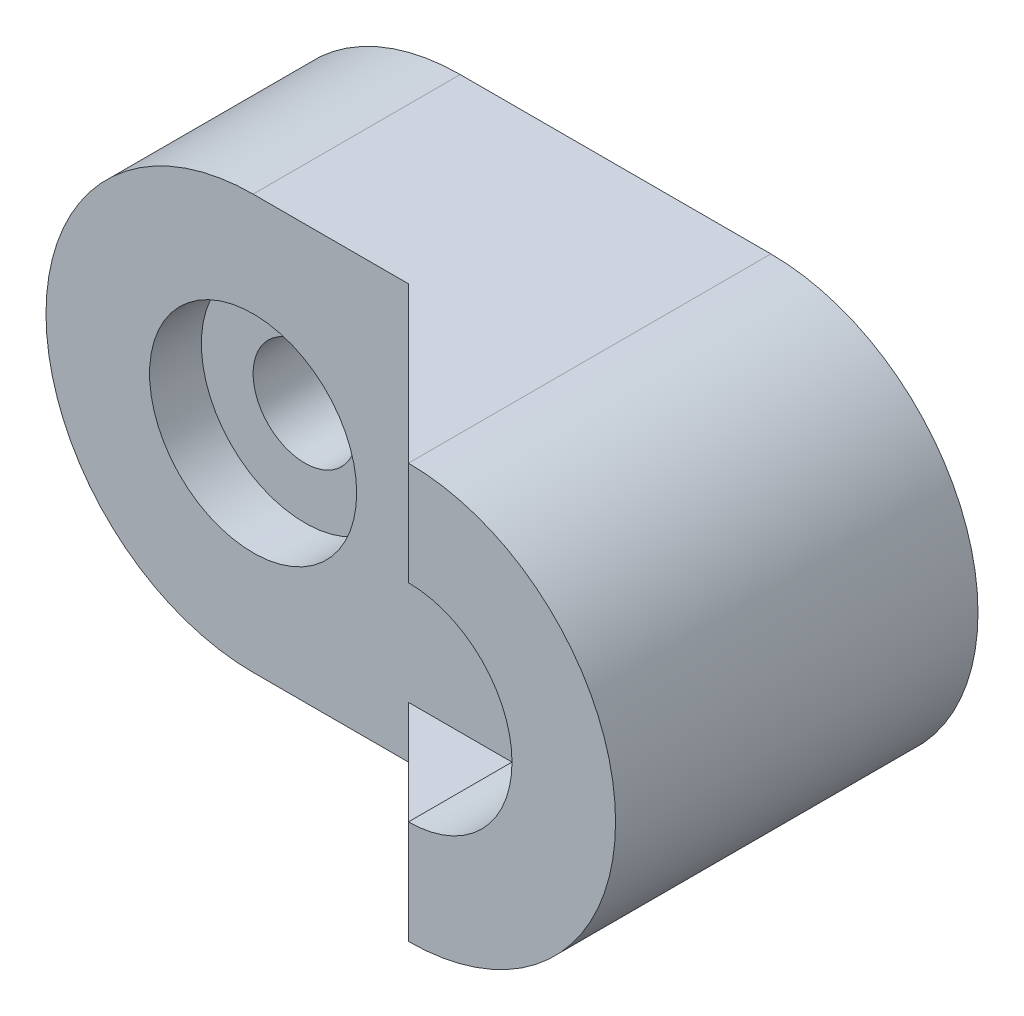
ISO-10303-21;
HEADER;
FILE_DESCRIPTION(('STEP AP214'),'2;1');
FILE_NAME('part.step','',(''),(''),'','','');
FILE_SCHEMA(('AUTOMOTIVE_DESIGN { 1 0 10303 214 1 1 1 1 }'));
ENDSEC;
DATA;
#1=APPLICATION_CONTEXT('core data for automotive mechanical design processes');
#2=APPLICATION_PROTOCOL_DEFINITION('international standard','automotive_design',2000,#1);
#3=PRODUCT_CONTEXT('',#1,'mechanical');
#4=PRODUCT('Part','Part','',(#3));
#5=PRODUCT_RELATED_PRODUCT_CATEGORY('part','',(#4));
#6=PRODUCT_DEFINITION_FORMATION('','',#4);
#7=PRODUCT_DEFINITION_CONTEXT('part definition',#1,'design');
#8=PRODUCT_DEFINITION('design','',#6,#7);
#9=PRODUCT_DEFINITION_SHAPE('','',#8);
#10=(LENGTH_UNIT() NAMED_UNIT(*) SI_UNIT(.MILLI.,.METRE.));
#11=(NAMED_UNIT(*) PLANE_ANGLE_UNIT() SI_UNIT($,.RADIAN.));
#12=(NAMED_UNIT(*) SI_UNIT($,.STERADIAN.) SOLID_ANGLE_UNIT());
#13=UNCERTAINTY_MEASURE_WITH_UNIT(LENGTH_MEASURE(1.E-05),#10,'distance_accuracy_value','');
#14=(GEOMETRIC_REPRESENTATION_CONTEXT(3) GLOBAL_UNCERTAINTY_ASSIGNED_CONTEXT((#13)) GLOBAL_UNIT_ASSIGNED_CONTEXT((#10,
#11,#12)) REPRESENTATION_CONTEXT('',''));
#15=CARTESIAN_POINT('',(0.,0.,0.));
#16=DIRECTION('',(0.,0.,1.));
#17=DIRECTION('',(1.,0.,0.));
#18=AXIS2_PLACEMENT_3D('',#15,#16,#17);
#19=CARTESIAN_POINT('',(60.,40.,70.));
#20=DIRECTION('',(1.,0.,0.));
#21=DIRECTION('',(0.,1.,0.));
#22=AXIS2_PLACEMENT_3D('',#19,#20,#21);
#23=PLANE('',#22);
#24=DIRECTION('',(0.,0.,-1.));
#25=VECTOR('',#24,1.);
#26=CARTESIAN_POINT('',(60.,30.,70.));
#27=LINE('',#26,#25);
#28=CARTESIAN_POINT('',(60.,30.,70.));
#29=VERTEX_POINT('',#28);
#30=CARTESIAN_POINT('',(60.,30.,40.));
#31=VERTEX_POINT('',#30);
#32=EDGE_CURVE('E127',#29,#31,#27,.T.);
#33=ORIENTED_EDGE('',*,*,#32,.T.);
#34=DIRECTION('',(0.,-1.,0.));
#35=VECTOR('',#34,1.);
#36=CARTESIAN_POINT('',(60.,40.,40.));
#37=LINE('',#36,#35);
#38=CARTESIAN_POINT('',(60.,20.,40.));
#39=VERTEX_POINT('',#38);
#40=EDGE_CURVE('E132',#31,#39,#37,.T.);
#41=ORIENTED_EDGE('',*,*,#40,.T.);
#42=DIRECTION('',(0.,0.,1.));
#43=VECTOR('',#42,1.);
#44=CARTESIAN_POINT('',(60.,20.,40.));
#45=LINE('',#44,#43);
#46=CARTESIAN_POINT('',(60.,20.,70.));
#47=VERTEX_POINT('',#46);
#48=EDGE_CURVE('E241',#39,#47,#45,.T.);
#49=ORIENTED_EDGE('',*,*,#48,.T.);
#50=DIRECTION('',(0.,-1.,0.));
#51=VECTOR('',#50,1.);
#52=CARTESIAN_POINT('',(60.,40.,70.));
#53=LINE('',#52,#51);
#54=EDGE_CURVE('E140',#29,#47,#53,.T.);
#55=ORIENTED_EDGE('',*,*,#54,.F.);
#56=EDGE_LOOP('',(#33,#41,#49,#55));
#57=FACE_BOUND('',#56,.T.);
#58=ADVANCED_FACE('F44',(#57),#23,.F.);
#59=CARTESIAN_POINT('',(0.,0.,40.));
#60=DIRECTION('',(0.,0.,-1.));
#61=DIRECTION('',(-1.,0.,0.));
#62=AXIS2_PLACEMENT_3D('',#59,#60,#61);
#63=CYLINDRICAL_SURFACE('',#62,40.);
#64=CARTESIAN_POINT('',(0.,0.,0.));
#65=DIRECTION('',(0.,0.,1.));
#66=DIRECTION('',(1.,0.,0.));
#67=AXIS2_PLACEMENT_3D('',#64,#65,#66);
#68=CIRCLE('',#67,40.);
#69=CARTESIAN_POINT('',(0.,40.,0.));
#70=VERTEX_POINT('',#69);
#71=CARTESIAN_POINT('',(0.,-40.,0.));
#72=VERTEX_POINT('',#71);
#73=EDGE_CURVE('E164',#70,#72,#68,.T.);
#74=ORIENTED_EDGE('',*,*,#73,.T.);
#75=DIRECTION('',(0.,0.,-1.));
#76=VECTOR('',#75,1.);
#77=CARTESIAN_POINT('',(0.,-40.,40.));
#78=LINE('',#77,#76);
#79=CARTESIAN_POINT('',(0.,-40.,40.));
#80=VERTEX_POINT('',#79);
#81=EDGE_CURVE('E11',#80,#72,#78,.T.);
#82=ORIENTED_EDGE('',*,*,#81,.F.);
#83=CARTESIAN_POINT('',(0.,0.,40.));
#84=DIRECTION('',(0.,0.,1.));
#85=DIRECTION('',(1.,0.,0.));
#86=AXIS2_PLACEMENT_3D('',#83,#84,#85);
#87=CIRCLE('',#86,40.);
#88=CARTESIAN_POINT('',(0.,40.,40.));
#89=VERTEX_POINT('',#88);
#90=EDGE_CURVE('E166',#89,#80,#87,.T.);
#91=ORIENTED_EDGE('',*,*,#90,.F.);
#92=DIRECTION('',(0.,0.,-1.));
#93=VECTOR('',#92,1.);
#94=CARTESIAN_POINT('',(0.,40.,40.));
#95=LINE('',#94,#93);
#96=EDGE_CURVE('E180',#89,#70,#95,.T.);
#97=ORIENTED_EDGE('',*,*,#96,.T.);
#98=EDGE_LOOP('',(#74,#82,#91,#97));
#99=FACE_BOUND('',#98,.T.);
#100=ADVANCED_FACE('F50',(#99),#63,.T.);
#101=CARTESIAN_POINT('',(60.,-40.,40.));
#102=DIRECTION('',(0.,1.,0.));
#103=DIRECTION('',(-1.,0.,0.));
#104=AXIS2_PLACEMENT_3D('',#101,#102,#103);
#105=PLANE('',#104);
#106=DIRECTION('',(1.,0.,0.));
#107=VECTOR('',#106,1.);
#108=CARTESIAN_POINT('',(60.,-40.,0.));
#109=LINE('',#108,#107);
#110=CARTESIAN_POINT('',(60.,-40.,0.));
#111=VERTEX_POINT('',#110);
#112=EDGE_CURVE('E179',#72,#111,#109,.T.);
#113=ORIENTED_EDGE('',*,*,#112,.T.);
#114=DIRECTION('',(0.,0.,-1.));
#115=VECTOR('',#114,1.);
#116=CARTESIAN_POINT('',(60.,-40.,40.));
#117=LINE('',#116,#115);
#118=CARTESIAN_POINT('',(60.,-40.,70.));
#119=VERTEX_POINT('',#118);
#120=EDGE_CURVE('E52',#119,#111,#117,.T.);
#121=ORIENTED_EDGE('',*,*,#120,.F.);
#122=DIRECTION('',(-0.707106781186547,0.,-0.707106781186548));
#123=VECTOR('',#122,1.);
#124=CARTESIAN_POINT('',(30.,-40.,40.));
#125=LINE('',#124,#123);
#126=CARTESIAN_POINT('',(30.,-40.,40.));
#127=VERTEX_POINT('',#126);
#128=EDGE_CURVE('E229',#119,#127,#125,.T.);
#129=ORIENTED_EDGE('',*,*,#128,.T.);
#130=DIRECTION('',(1.,0.,0.));
#131=VECTOR('',#130,1.);
#132=CARTESIAN_POINT('',(60.,-40.,40.));
#133=LINE('',#132,#131);
#134=EDGE_CURVE('E171',#80,#127,#133,.T.);
#135=ORIENTED_EDGE('',*,*,#134,.F.);
#136=ORIENTED_EDGE('',*,*,#81,.T.);
#137=EDGE_LOOP('',(#113,#121,#129,#135,#136));
#138=FACE_BOUND('',#137,.T.);
#139=ADVANCED_FACE('F257',(#138),#105,.F.);
#140=CARTESIAN_POINT('',(60.,0.,40.));
#141=DIRECTION('',(0.,0.,-1.));
#142=DIRECTION('',(-1.,0.,0.));
#143=AXIS2_PLACEMENT_3D('',#140,#141,#142);
#144=CYLINDRICAL_SURFACE('',#143,40.);
#145=CARTESIAN_POINT('',(60.,0.,0.));
#146=DIRECTION('',(0.,0.,1.));
#147=DIRECTION('',(1.,0.,0.));
#148=AXIS2_PLACEMENT_3D('',#145,#146,#147);
#149=CIRCLE('',#148,40.);
#150=CARTESIAN_POINT('',(60.,40.,0.));
#151=VERTEX_POINT('',#150);
#152=EDGE_CURVE('E185',#111,#151,#149,.T.);
#153=ORIENTED_EDGE('',*,*,#152,.T.);
#154=DIRECTION('',(0.,0.,-1.));
#155=VECTOR('',#154,1.);
#156=CARTESIAN_POINT('',(60.,40.,40.));
#157=LINE('',#156,#155);
#158=CARTESIAN_POINT('',(60.,40.,70.));
#159=VERTEX_POINT('',#158);
#160=EDGE_CURVE('E190',#159,#151,#157,.T.);
#161=ORIENTED_EDGE('',*,*,#160,.F.);
#162=CARTESIAN_POINT('',(60.,0.,70.));
#163=DIRECTION('',(0.,0.,1.));
#164=DIRECTION('',(1.,0.,0.));
#165=AXIS2_PLACEMENT_3D('',#162,#163,#164);
#166=CIRCLE('',#165,40.);
#167=EDGE_CURVE('E143',#119,#159,#166,.T.);
#168=ORIENTED_EDGE('',*,*,#167,.F.);
#169=ORIENTED_EDGE('',*,*,#120,.T.);
#170=EDGE_LOOP('',(#153,#161,#168,#169));
#171=FACE_BOUND('',#170,.T.);
#172=ADVANCED_FACE('F194',(#171),#144,.T.);
#173=CARTESIAN_POINT('',(0.,40.,40.));
#174=DIRECTION('',(0.,-1.,0.));
#175=DIRECTION('',(1.,0.,0.));
#176=AXIS2_PLACEMENT_3D('',#173,#174,#175);
#177=PLANE('',#176);
#178=DIRECTION('',(-1.,0.,0.));
#179=VECTOR('',#178,1.);
#180=CARTESIAN_POINT('',(0.,40.,0.));
#181=LINE('',#180,#179);
#182=EDGE_CURVE('E175',#151,#70,#181,.T.);
#183=ORIENTED_EDGE('',*,*,#182,.T.);
#184=ORIENTED_EDGE('',*,*,#96,.F.);
#185=DIRECTION('',(-1.,0.,0.));
#186=VECTOR('',#185,1.);
#187=CARTESIAN_POINT('',(0.,40.,40.));
#188=LINE('',#187,#186);
#189=CARTESIAN_POINT('',(30.,40.,40.));
#190=VERTEX_POINT('',#189);
#191=EDGE_CURVE('E174',#190,#89,#188,.T.);
#192=ORIENTED_EDGE('',*,*,#191,.F.);
#193=DIRECTION('',(0.707106781186547,0.,0.707106781186548));
#194=VECTOR('',#193,1.);
#195=CARTESIAN_POINT('',(30.,40.,40.));
#196=LINE('',#195,#194);
#197=EDGE_CURVE('E208',#190,#159,#196,.T.);
#198=ORIENTED_EDGE('',*,*,#197,.T.);
#199=ORIENTED_EDGE('',*,*,#160,.T.);
#200=EDGE_LOOP('',(#183,#184,#192,#198,#199));
#201=FACE_BOUND('',#200,.T.);
#202=ADVANCED_FACE('F203',(#201),#177,.F.);
#203=CARTESIAN_POINT('',(0.,0.,40.));
#204=DIRECTION('',(0.,0.,1.));
#205=DIRECTION('',(1.,0.,0.));
#206=AXIS2_PLACEMENT_3D('',#203,#204,#205);
#207=PLANE('',#206);
#208=DIRECTION('',(0.,1.,0.));
#209=VECTOR('',#208,1.);
#210=CARTESIAN_POINT('',(30.,30.,40.));
#211=LINE('',#210,#209);
#212=CARTESIAN_POINT('',(30.,30.,40.));
#213=VERTEX_POINT('',#212);
#214=EDGE_CURVE('E133',#213,#190,#211,.T.);
#215=ORIENTED_EDGE('',*,*,#214,.T.);
#216=ORIENTED_EDGE('',*,*,#191,.T.);
#217=ORIENTED_EDGE('',*,*,#90,.T.);
#218=ORIENTED_EDGE('',*,*,#134,.T.);
#219=DIRECTION('',(0.,-1.,0.));
#220=VECTOR('',#219,1.);
#221=CARTESIAN_POINT('',(30.,-30.,40.));
#222=LINE('',#221,#220);
#223=CARTESIAN_POINT('',(30.,-30.,40.));
#224=VERTEX_POINT('',#223);
#225=EDGE_CURVE('E225',#224,#127,#222,.T.);
#226=ORIENTED_EDGE('',*,*,#225,.F.);
#227=DIRECTION('',(1.,0.,0.));
#228=VECTOR('',#227,1.);
#229=CARTESIAN_POINT('',(60.,-30.,40.));
#230=LINE('',#229,#228);
#231=CARTESIAN_POINT('',(60.,-30.,40.));
#232=VERTEX_POINT('',#231);
#233=EDGE_CURVE('E249',#224,#232,#230,.T.);
#234=ORIENTED_EDGE('',*,*,#233,.T.);
#235=CARTESIAN_POINT('',(60.,-20.,40.));
#236=VERTEX_POINT('',#235);
#237=EDGE_CURVE('E147',#236,#232,#37,.T.);
#238=ORIENTED_EDGE('',*,*,#237,.F.);
#239=CARTESIAN_POINT('',(60.,0.,40.));
#240=DIRECTION('',(0.,0.,1.));
#241=DIRECTION('',(1.,0.,0.));
#242=AXIS2_PLACEMENT_3D('',#239,#240,#241);
#243=CIRCLE('',#242,20.);
#244=EDGE_CURVE('E141',#39,#236,#243,.T.);
#245=ORIENTED_EDGE('',*,*,#244,.F.);
#246=ORIENTED_EDGE('',*,*,#40,.F.);
#247=DIRECTION('',(-1.,0.,0.));
#248=VECTOR('',#247,1.);
#249=CARTESIAN_POINT('',(60.,30.,40.));
#250=LINE('',#249,#248);
#251=EDGE_CURVE('E124',#31,#213,#250,.T.);
#252=ORIENTED_EDGE('',*,*,#251,.T.);
#253=EDGE_LOOP('',(#215,#216,#217,#218,#226,#234,#238,#245,#246,#252));
#254=FACE_BOUND('',#253,.T.);
#255=CARTESIAN_POINT('',(0.,0.,40.));
#256=DIRECTION('',(0.,0.,1.));
#257=DIRECTION('',(1.,0.,0.));
#258=AXIS2_PLACEMENT_3D('',#255,#256,#257);
#259=CIRCLE('',#258,20.);
#260=CARTESIAN_POINT('',(20.,0.,40.));
#261=VERTEX_POINT('',#260);
#262=EDGE_CURVE('E158',#261,#261,#259,.T.);
#263=ORIENTED_EDGE('',*,*,#262,.F.);
#264=EDGE_LOOP('',(#263));
#265=FACE_BOUND('',#264,.T.);
#266=ADVANCED_FACE('F136',(#254,#265),#207,.T.);
#267=CARTESIAN_POINT('',(0.,0.,0.));
#268=DIRECTION('',(0.,0.,1.));
#269=DIRECTION('',(1.,0.,0.));
#270=AXIS2_PLACEMENT_3D('',#267,#268,#269);
#271=PLANE('',#270);
#272=CARTESIAN_POINT('',(60.,0.,0.));
#273=DIRECTION('',(0.,0.,1.));
#274=DIRECTION('',(1.,0.,0.));
#275=AXIS2_PLACEMENT_3D('',#272,#273,#274);
#276=CIRCLE('',#275,9.99999999999999);
#277=CARTESIAN_POINT('',(70.,0.,0.));
#278=VERTEX_POINT('',#277);
#279=EDGE_CURVE('E221',#278,#278,#276,.T.);
#280=ORIENTED_EDGE('',*,*,#279,.T.);
#281=EDGE_LOOP('',(#280));
#282=FACE_BOUND('',#281,.T.);
#283=CARTESIAN_POINT('',(0.,0.,0.));
#284=DIRECTION('',(0.,0.,1.));
#285=DIRECTION('',(1.,0.,0.));
#286=AXIS2_PLACEMENT_3D('',#283,#284,#285);
#287=CIRCLE('',#286,10.);
#288=CARTESIAN_POINT('',(10.,0.,0.));
#289=VERTEX_POINT('',#288);
#290=EDGE_CURVE('E152',#289,#289,#287,.T.);
#291=ORIENTED_EDGE('',*,*,#290,.T.);
#292=EDGE_LOOP('',(#291));
#293=FACE_BOUND('',#292,.T.);
#294=ORIENTED_EDGE('',*,*,#73,.F.);
#295=ORIENTED_EDGE('',*,*,#182,.F.);
#296=ORIENTED_EDGE('',*,*,#152,.F.);
#297=ORIENTED_EDGE('',*,*,#112,.F.);
#298=EDGE_LOOP('',(#294,#295,#296,#297));
#299=FACE_BOUND('',#298,.T.);
#300=ADVANCED_FACE('F197',(#282,#293,#299),#271,.F.);
#301=CARTESIAN_POINT('',(0.,0.,30.));
#302=DIRECTION('',(0.,0.,1.));
#303=DIRECTION('',(1.,0.,0.));
#304=AXIS2_PLACEMENT_3D('',#301,#302,#303);
#305=CYLINDRICAL_SURFACE('',#304,20.);
#306=CARTESIAN_POINT('',(0.,0.,30.));
#307=DIRECTION('',(0.,0.,1.));
#308=DIRECTION('',(1.,0.,0.));
#309=AXIS2_PLACEMENT_3D('',#306,#307,#308);
#310=CIRCLE('',#309,20.);
#311=CARTESIAN_POINT('',(20.,0.,30.));
#312=VERTEX_POINT('',#311);
#313=EDGE_CURVE('E162',#312,#312,#310,.T.);
#314=ORIENTED_EDGE('',*,*,#313,.F.);
#315=EDGE_LOOP('',(#314));
#316=FACE_BOUND('',#315,.T.);
#317=ORIENTED_EDGE('',*,*,#262,.T.);
#318=EDGE_LOOP('',(#317));
#319=FACE_BOUND('',#318,.T.);
#320=ADVANCED_FACE('F292',(#316,#319),#305,.F.);
#321=CARTESIAN_POINT('',(0.,0.,30.));
#322=DIRECTION('',(0.,0.,1.));
#323=DIRECTION('',(1.,0.,0.));
#324=AXIS2_PLACEMENT_3D('',#321,#322,#323);
#325=PLANE('',#324);
#326=CARTESIAN_POINT('',(0.,0.,30.));
#327=DIRECTION('',(0.,0.,1.));
#328=DIRECTION('',(1.,0.,0.));
#329=AXIS2_PLACEMENT_3D('',#326,#327,#328);
#330=CIRCLE('',#329,10.);
#331=CARTESIAN_POINT('',(10.,0.,30.));
#332=VERTEX_POINT('',#331);
#333=EDGE_CURVE('E159',#332,#332,#330,.T.);
#334=ORIENTED_EDGE('',*,*,#333,.F.);
#335=EDGE_LOOP('',(#334));
#336=FACE_BOUND('',#335,.T.);
#337=ORIENTED_EDGE('',*,*,#313,.T.);
#338=EDGE_LOOP('',(#337));
#339=FACE_BOUND('',#338,.T.);
#340=ADVANCED_FACE('F287',(#336,#339),#325,.T.);
#341=CARTESIAN_POINT('',(0.,0.,0.));
#342=DIRECTION('',(0.,0.,1.));
#343=DIRECTION('',(1.,0.,0.));
#344=AXIS2_PLACEMENT_3D('',#341,#342,#343);
#345=CYLINDRICAL_SURFACE('',#344,10.);
#346=ORIENTED_EDGE('',*,*,#290,.F.);
#347=EDGE_LOOP('',(#346));
#348=FACE_BOUND('',#347,.T.);
#349=ORIENTED_EDGE('',*,*,#333,.T.);
#350=EDGE_LOOP('',(#349));
#351=FACE_BOUND('',#350,.T.);
#352=ADVANCED_FACE('F276',(#348,#351),#345,.F.);
#353=ORIENTED_EDGE('',*,*,#237,.T.);
#354=DIRECTION('',(0.,0.,1.));
#355=VECTOR('',#354,1.);
#356=CARTESIAN_POINT('',(60.,-30.,70.));
#357=LINE('',#356,#355);
#358=CARTESIAN_POINT('',(60.,-30.,70.));
#359=VERTEX_POINT('',#358);
#360=EDGE_CURVE('E227',#232,#359,#357,.T.);
#361=ORIENTED_EDGE('',*,*,#360,.T.);
#362=CARTESIAN_POINT('',(60.,-20.,70.));
#363=VERTEX_POINT('',#362);
#364=EDGE_CURVE('E146',#363,#359,#53,.T.);
#365=ORIENTED_EDGE('',*,*,#364,.F.);
#366=DIRECTION('',(0.,0.,1.));
#367=VECTOR('',#366,1.);
#368=CARTESIAN_POINT('',(60.,-20.,40.));
#369=LINE('',#368,#367);
#370=EDGE_CURVE('E66',#236,#363,#369,.T.);
#371=ORIENTED_EDGE('',*,*,#370,.F.);
#372=EDGE_LOOP('',(#353,#361,#365,#371));
#373=FACE_BOUND('',#372,.T.);
#374=ADVANCED_FACE('F250',(#373),#23,.F.);
#375=CARTESIAN_POINT('',(60.,0.,70.));
#376=DIRECTION('',(0.,0.,1.));
#377=DIRECTION('',(1.,0.,0.));
#378=AXIS2_PLACEMENT_3D('',#375,#376,#377);
#379=PLANE('',#378);
#380=CARTESIAN_POINT('',(60.,0.,70.));
#381=DIRECTION('',(0.,0.,1.));
#382=DIRECTION('',(1.,0.,0.));
#383=AXIS2_PLACEMENT_3D('',#380,#381,#382);
#384=CIRCLE('',#383,20.);
#385=EDGE_CURVE('E238',#363,#47,#384,.T.);
#386=ORIENTED_EDGE('',*,*,#385,.F.);
#387=ORIENTED_EDGE('',*,*,#364,.T.);
#388=DIRECTION('',(0.,-1.,0.));
#389=VECTOR('',#388,1.);
#390=CARTESIAN_POINT('',(60.,-30.,70.));
#391=LINE('',#390,#389);
#392=EDGE_CURVE('E218',#359,#119,#391,.T.);
#393=ORIENTED_EDGE('',*,*,#392,.T.);
#394=ORIENTED_EDGE('',*,*,#167,.T.);
#395=EDGE_CURVE('E154',#159,#29,#53,.T.);
#396=ORIENTED_EDGE('',*,*,#395,.T.);
#397=ORIENTED_EDGE('',*,*,#54,.T.);
#398=EDGE_LOOP('',(#386,#387,#393,#394,#396,#397));
#399=FACE_BOUND('',#398,.T.);
#400=ADVANCED_FACE('F211',(#399),#379,.T.);
#401=CARTESIAN_POINT('',(60.,0.,40.));
#402=DIRECTION('',(0.,0.,1.));
#403=DIRECTION('',(1.,0.,0.));
#404=AXIS2_PLACEMENT_3D('',#401,#402,#403);
#405=CYLINDRICAL_SURFACE('',#404,20.);
#406=ORIENTED_EDGE('',*,*,#385,.T.);
#407=ORIENTED_EDGE('',*,*,#48,.F.);
#408=ORIENTED_EDGE('',*,*,#244,.T.);
#409=ORIENTED_EDGE('',*,*,#370,.T.);
#410=EDGE_LOOP('',(#406,#407,#408,#409));
#411=FACE_BOUND('',#410,.T.);
#412=CARTESIAN_POINT('',(60.,0.,30.));
#413=DIRECTION('',(0.,0.,1.));
#414=DIRECTION('',(1.,0.,0.));
#415=AXIS2_PLACEMENT_3D('',#412,#413,#414);
#416=CIRCLE('',#415,20.);
#417=CARTESIAN_POINT('',(80.,0.,30.));
#418=VERTEX_POINT('',#417);
#419=EDGE_CURVE('E232',#418,#418,#416,.T.);
#420=ORIENTED_EDGE('',*,*,#419,.F.);
#421=EDGE_LOOP('',(#420));
#422=FACE_BOUND('',#421,.T.);
#423=ADVANCED_FACE('F243',(#411,#422),#405,.F.);
#424=CARTESIAN_POINT('',(60.,0.,30.));
#425=DIRECTION('',(0.,0.,1.));
#426=DIRECTION('',(1.,0.,0.));
#427=AXIS2_PLACEMENT_3D('',#424,#425,#426);
#428=PLANE('',#427);
#429=CARTESIAN_POINT('',(60.,0.,30.));
#430=DIRECTION('',(0.,0.,1.));
#431=DIRECTION('',(1.,0.,0.));
#432=AXIS2_PLACEMENT_3D('',#429,#430,#431);
#433=CIRCLE('',#432,9.99999999999999);
#434=CARTESIAN_POINT('',(70.,0.,30.));
#435=VERTEX_POINT('',#434);
#436=EDGE_CURVE('E222',#435,#435,#433,.T.);
#437=ORIENTED_EDGE('',*,*,#436,.F.);
#438=EDGE_LOOP('',(#437));
#439=FACE_BOUND('',#438,.T.);
#440=ORIENTED_EDGE('',*,*,#419,.T.);
#441=EDGE_LOOP('',(#440));
#442=FACE_BOUND('',#441,.T.);
#443=ADVANCED_FACE('F318',(#439,#442),#428,.T.);
#444=CARTESIAN_POINT('',(60.,0.,0.));
#445=DIRECTION('',(0.,0.,1.));
#446=DIRECTION('',(1.,0.,0.));
#447=AXIS2_PLACEMENT_3D('',#444,#445,#446);
#448=CYLINDRICAL_SURFACE('',#447,9.99999999999999);
#449=ORIENTED_EDGE('',*,*,#279,.F.);
#450=EDGE_LOOP('',(#449));
#451=FACE_BOUND('',#450,.T.);
#452=ORIENTED_EDGE('',*,*,#436,.T.);
#453=EDGE_LOOP('',(#452));
#454=FACE_BOUND('',#453,.T.);
#455=ADVANCED_FACE('F270',(#451,#454),#448,.F.);
#456=CARTESIAN_POINT('',(30.,-30.,40.));
#457=DIRECTION('',(-0.707106781186548,0.,0.707106781186547));
#458=DIRECTION('',(0.707106781186547,0.,0.707106781186548));
#459=AXIS2_PLACEMENT_3D('',#456,#457,#458);
#460=PLANE('',#459);
#461=ORIENTED_EDGE('',*,*,#128,.F.);
#462=ORIENTED_EDGE('',*,*,#392,.F.);
#463=DIRECTION('',(-0.707106781186547,0.,-0.707106781186548));
#464=VECTOR('',#463,1.);
#465=CARTESIAN_POINT('',(30.,-30.,40.));
#466=LINE('',#465,#464);
#467=EDGE_CURVE('E252',#359,#224,#466,.T.);
#468=ORIENTED_EDGE('',*,*,#467,.T.);
#469=ORIENTED_EDGE('',*,*,#225,.T.);
#470=EDGE_LOOP('',(#461,#462,#468,#469));
#471=FACE_BOUND('',#470,.T.);
#472=ADVANCED_FACE('F260',(#471),#460,.T.);
#473=CARTESIAN_POINT('',(0.,-30.,0.));
#474=DIRECTION('',(0.,1.,0.));
#475=DIRECTION('',(-1.,0.,0.));
#476=AXIS2_PLACEMENT_3D('',#473,#474,#475);
#477=PLANE('',#476);
#478=ORIENTED_EDGE('',*,*,#467,.F.);
#479=ORIENTED_EDGE('',*,*,#360,.F.);
#480=ORIENTED_EDGE('',*,*,#233,.F.);
#481=EDGE_LOOP('',(#478,#479,#480));
#482=FACE_BOUND('',#481,.T.);
#483=ADVANCED_FACE('F259',(#482),#477,.T.);
#484=CARTESIAN_POINT('',(30.,30.,40.));
#485=DIRECTION('',(-0.707106781186548,0.,0.707106781186547));
#486=DIRECTION('',(0.707106781186547,0.,0.707106781186548));
#487=AXIS2_PLACEMENT_3D('',#484,#485,#486);
#488=PLANE('',#487);
#489=ORIENTED_EDGE('',*,*,#197,.F.);
#490=ORIENTED_EDGE('',*,*,#214,.F.);
#491=DIRECTION('',(0.707106781186547,0.,0.707106781186548));
#492=VECTOR('',#491,1.);
#493=CARTESIAN_POINT('',(30.,30.,40.));
#494=LINE('',#493,#492);
#495=EDGE_CURVE('E58',#213,#29,#494,.T.);
#496=ORIENTED_EDGE('',*,*,#495,.T.);
#497=ORIENTED_EDGE('',*,*,#395,.F.);
#498=EDGE_LOOP('',(#489,#490,#496,#497));
#499=FACE_BOUND('',#498,.T.);
#500=ADVANCED_FACE('F258',(#499),#488,.T.);
#501=CARTESIAN_POINT('',(0.,30.,0.));
#502=DIRECTION('',(0.,1.,0.));
#503=DIRECTION('',(-1.,0.,0.));
#504=AXIS2_PLACEMENT_3D('',#501,#502,#503);
#505=PLANE('',#504);
#506=ORIENTED_EDGE('',*,*,#495,.F.);
#507=ORIENTED_EDGE('',*,*,#251,.F.);
#508=ORIENTED_EDGE('',*,*,#32,.F.);
#509=EDGE_LOOP('',(#506,#507,#508));
#510=FACE_BOUND('',#509,.T.);
#511=ADVANCED_FACE('F123',(#510),#505,.F.);
#512=CLOSED_SHELL('',(#58,#100,#139,#172,#202,#266,#300,#320,#340,#352,#374,#400,#423,#443,#455,
#472,#483,#500,#511));
#513=MANIFOLD_SOLID_BREP('B2',#512);
#514=ADVANCED_BREP_SHAPE_REPRESENTATION('',(#18,#513),#14);
#515=SHAPE_DEFINITION_REPRESENTATION(#9,#514);
ENDSEC;
END-ISO-10303-21;
